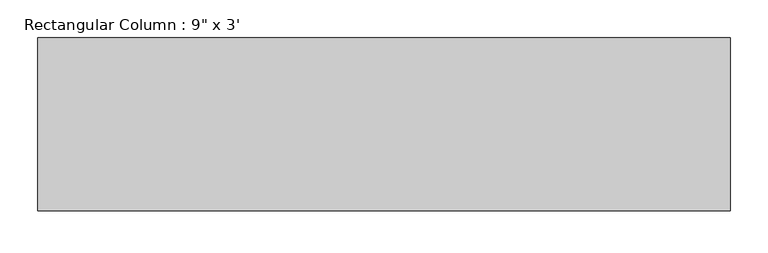
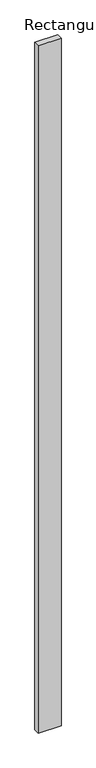
"""IFC4 building model written with IfcOpenShell, lengths in millimetres: column geometry."""

from ifc_helpers import new_model, si_unit, origin, origin_with_axes, place, context, project, spatial, polyline, outline, extrude, source, transform, mapped, element, save


def column_35a9bf28(model_context):
    return source(origin(), model_context, "Body", "SweptSolid", [
        extrude(outline(polyline([(457.2, 114.3), (457.2, -114.3), (-457.2, -114.3), (-457.2, 114.3), (457.2, 114.3)])), origin_with_axes(), (0.0, 0.0, 1.0), 29108.4),
    ])


if __name__ == "__main__":
    model = new_model("IFC4")
    model_context = context("Model", 3, world=origin())
    ifc_project = project(units=[si_unit("LENGTHUNIT", "METRE", prefix="MILLI")], contexts=[model_context])
    site = spatial("IfcSite", under=ifc_project)
    building = spatial("IfcBuilding", under=site)
    placement = place(None, origin())
    column_shape = column_35a9bf28(model_context)
    element("IfcColumn", 1, ObjectType="Rectangular Column : 9\" x 3'", at=placement, inside=building, context=model_context, shape_type="MappedRepresentation", body=[
        mapped(column_shape, transform((0.0, 0.0, 0.0), x_axis=(1.0, 0.0, 0.0), y_axis=(0.0, 1.0, 0.0), z_axis=(0.0, 0.0, 1.0))),
    ])
    save(model, "model.ifc")

# Revit data of these elements
# Type "Rectangular Column : 9\" x 3'"
#   Assembly Code = "B1010200"
#   Depth = 0' - 9"
#   Offset Base = 0' - 0"
#   Offset Top = 0' - 0"
#   Width = 3' - 0"
#   Material = none
